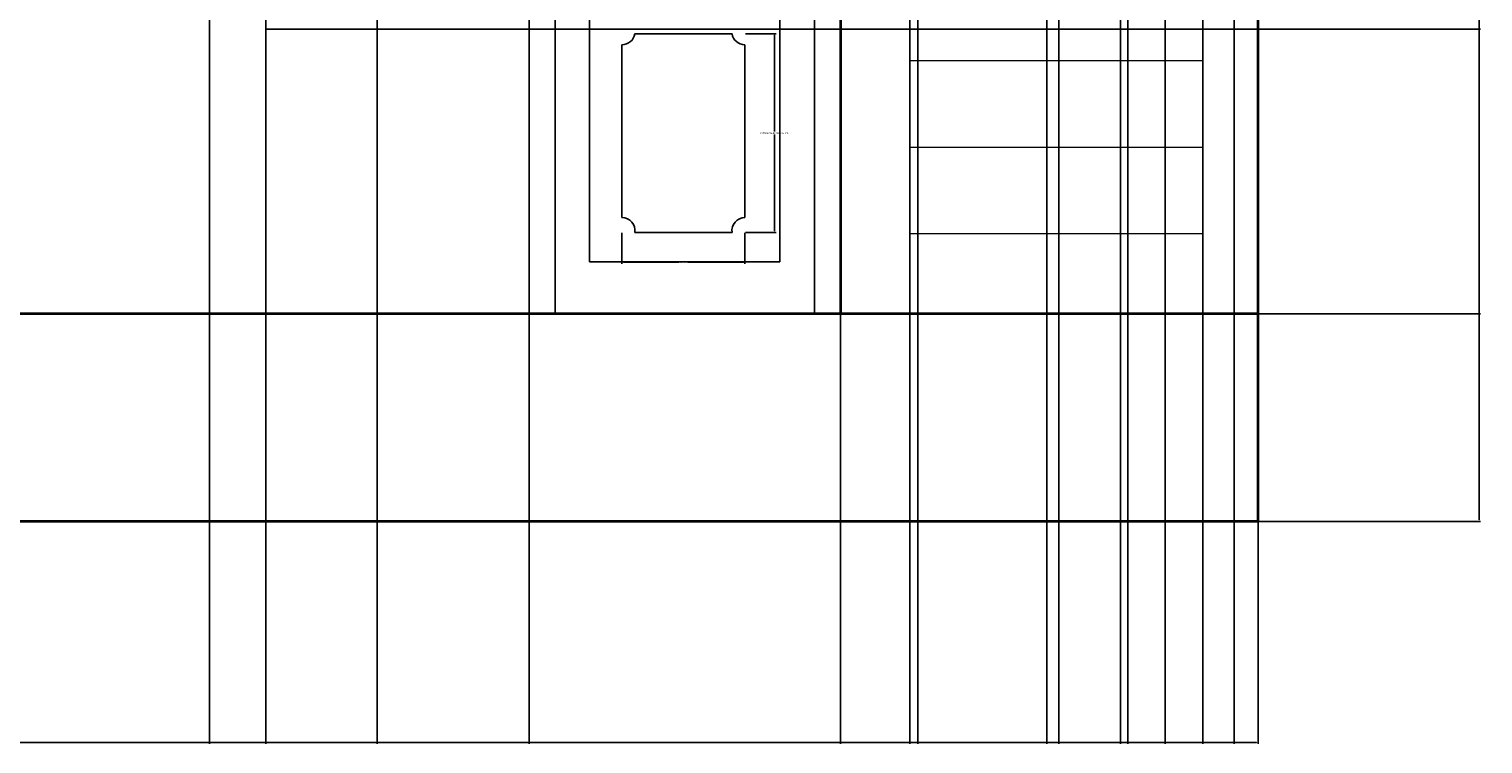
# Model space of a CAD drawing. Units: inches. Extents: x 93 to 565, y 123 to 656.
# Tile 3 of 18: x 397 to 565, y 134 to 217. Entities that reach past the tile are written whole.
import ezdxf

# ---------------------------------------------------------------- set-up
doc = ezdxf.new("R2010")
doc.units = ezdxf.units.IN
doc.header["$MEASUREMENT"] = 0
for name, color, linetype, lineweight in [('A-ANNO-DIMS', 2, 'Continuous', 18), ('A-DOOR', 3, 'Continuous', 25), ('A-ELEV', 7, 'Continuous', 35), ('A-FLOR-STRS', 6, 'Continuous', 18)]:
    doc.layers.add(name, color=color, linetype=linetype, lineweight=lineweight)
doc.styles.get("Standard").update_dxf_attribs({"font": 'arial.ttf'})
doc.dimstyles.get("Standard").update_dxf_attribs({"dimtxt": 0.18, "dimasz": 0.18, "dimexe": 0.18, "dimexo": 0.0625, "dimgap": 0.09, "dimtad": 0, "dimtih": 1, "dimtoh": 1, "dimdec": 4, "dimzin": 0, "dimdsep": 46, "dimtxsty": 'Standard', "dimcen": 0.09, "dimadec": 0, "dimazin": 0, "dimtfac": 1, "dimtdec": 4, "dimtofl": 0, "dimtmove": 0, "dimatfit": 3, "dimfxl": 1, "dimtolj": 1, "dimtzin": 0, "dimarcsym": 0})

# ---------------------------------------------------------------- blocks, each defined once
blk = doc.blocks.new('*U4')
blk.add_lwpolyline([(3.12, 0.01), (0.12, 0.01), (0.12, 84.01), (36.12, 84.01), (36.12, 0.01), (33.12, 0.01)])
for points in [[(33.12, 80.99), (33.12, 0.01), (3.12, 0.01), (3.12, 80.99)], [(29.12, 6.01), (29.12, 74.99), (7.12, 74.99), (7.12, 6.01)]]:
    blk.add_lwpolyline(points, close=True)
blk.add_circle((31.12, 42.01), 1)
blk = doc.blocks.new('DOOR-PANEL-LOWER')
for points in [[(1.48, 22.97), (12.73, 22.97)], [(0, 1.72), (0, 21.69)], [(14.21, 21.69), (14.21, 1.72)], [(12.73, 0), (1.48, 0)]]:
    blk.add_lwpolyline(points)
for centre, start, end in [((0, 23.19), 270, 351.5859), ((14.21, 23.19), 188.4141, 270), ((0, 0.22), 351.5859, 90), ((14.21, 0.22), 90, 188.4141)]:
    blk.add_arc(centre, 1.5, start, end)
blk = doc.blocks.new('*D24')
at = {"layer": 'A-ANNO-DIMS', "color": 0, "lineweight": -2, "transparency": 16777216}
for p, q in [((479.78, 216.1), (483.34, 216.1)), ((483.16, 215.92), (483.16, 204.79)), ((483.16, 193.3), (483.16, 204.43)), ((479.78, 193.12), (483.34, 193.12))]:
    blk.add_line(p, q, dxfattribs=at)
at = {"layer": 'A-ANNO-DIMS', "color": 0, "transparency": 16777216}
for points in [[(483.13, 215.92), (483.19, 215.92), (483.16, 216.1)], [(483.13, 193.3), (483.19, 193.3), (483.16, 193.12)]]:
    blk.add_solid(points, dxfattribs=at)
at = {"layer": 'Defpoints', "color": 0, "transparency": 16777216}
for p in [(479.72, 216.1), (483.16, 216.1), (479.72, 193.12)]:
    blk.add_point(p, dxfattribs=at)
at = {"layer": 'A-ANNO-DIMS', "color": 0, "transparency": 16777216, "insert": (483.16, 204.61), "char_height": 0.18, "attachment_point": 5}
blk.add_mtext('\\A1;DOOR LOWER PANEL 23 TYP.', dxfattribs=at)
blk = doc.blocks.new('*D25')
at = {"layer": 'A-ANNO-DIMS', "color": 0, "lineweight": -2, "transparency": 16777216}
for p, q in [((465.5, 193.06), (465.5, 189.5)), ((479.72, 193.06), (479.72, 189.5)), ((465.68, 189.68), (472.09, 189.68)), ((479.54, 189.68), (473.13, 189.68))]:
    blk.add_line(p, q, dxfattribs=at)
at = {"layer": 'A-ANNO-DIMS', "color": 0, "transparency": 16777216}
for points in [[(465.68, 189.71), (465.68, 189.65), (465.5, 189.68)], [(479.54, 189.71), (479.54, 189.65), (479.72, 189.68)]]:
    blk.add_solid(points, dxfattribs=at)
at = {"layer": 'Defpoints', "color": 0, "transparency": 16777216}
for p in [(465.5, 193.12), (479.72, 193.12), (479.72, 189.68)]:
    blk.add_point(p, dxfattribs=at)
at = {"layer": 'A-ANNO-DIMS', "color": 0, "transparency": 16777216, "insert": (472.61, 189.68), "char_height": 0.18, "attachment_point": 5}
blk.add_mtext('\\A1;14 TYP.', dxfattribs=at)
blk = doc.blocks.new('*D29')
at = {"layer": 'A-ANNO-DIMS', "color": 0, "lineweight": -2, "transparency": 16777216}
for p, q in [((437.19, 594.34), (437.19, 134)), ((295.69, 183.67), (295.69, 134)), ((295.87, 134.18), (366.05, 134.18)), ((437.01, 134.18), (366.82, 134.18))]:
    blk.add_line(p, q, dxfattribs=at)
at = {"layer": 'A-ANNO-DIMS', "color": 0, "transparency": 16777216}
for points in [[(295.87, 134.21), (295.87, 134.15), (295.69, 134.18)], [(437.01, 134.21), (437.01, 134.15), (437.19, 134.18)]]:
    blk.add_solid(points, dxfattribs=at)
at = {"layer": 'Defpoints', "color": 0, "transparency": 16777216}
for p in [(437.19, 594.4), (295.69, 183.73), (437.19, 134.18)]:
    blk.add_point(p, dxfattribs=at)
at = {"layer": 'A-ANNO-DIMS', "color": 0, "transparency": 16777216, "insert": (366.44, 134.18), "char_height": 0.18, "attachment_point": 5}
blk.add_mtext('\\A1;141.5', dxfattribs=at)
blk = doc.blocks.new('*D30')
at = {"layer": 'A-ANNO-DIMS', "color": 0, "lineweight": -2, "transparency": 16777216}
for p, q in [((437.19, 594.34), (437.19, 134)), ((539.08, 159.67), (539.08, 134)), ((437.37, 134.18), (487.75, 134.18)), ((538.9, 134.18), (488.52, 134.18))]:
    blk.add_line(p, q, dxfattribs=at)
at = {"layer": 'A-ANNO-DIMS', "color": 0, "transparency": 16777216}
for points in [[(437.37, 134.21), (437.37, 134.15), (437.19, 134.18)], [(538.9, 134.21), (538.9, 134.15), (539.08, 134.18)]]:
    blk.add_solid(points, dxfattribs=at)
at = {"layer": 'Defpoints', "color": 0, "transparency": 16777216}
for p in [(437.19, 594.4), (539.08, 159.73), (539.08, 134.18)]:
    blk.add_point(p, dxfattribs=at)
at = {"layer": 'A-ANNO-DIMS', "color": 0, "transparency": 16777216, "insert": (488.13, 134.18), "char_height": 0.18, "attachment_point": 5}
blk.add_mtext('\\A1;101.9', dxfattribs=at)
blk = doc.blocks.new('*D31')
at = {"layer": 'A-ANNO-DIMS', "color": 0, "lineweight": -2, "transparency": 16777216}
for p, q in [((417.87, 630.4), (564.81, 630.4)), ((564.63, 630.22), (564.63, 395.25)), ((564.63, 159.91), (564.63, 394.89)), ((119.14, 159.73), (564.81, 159.73))]:
    blk.add_line(p, q, dxfattribs=at)
at = {"layer": 'A-ANNO-DIMS', "color": 0, "transparency": 16777216}
for points in [[(564.6, 630.22), (564.66, 630.22), (564.63, 630.4)], [(564.6, 159.91), (564.66, 159.91), (564.63, 159.73)]]:
    blk.add_solid(points, dxfattribs=at)
at = {"layer": 'Defpoints', "color": 0, "transparency": 16777216}
for p in [(417.81, 630.4), (564.63, 630.4), (119.08, 159.73)]:
    blk.add_point(p, dxfattribs=at)
at = {"layer": 'A-ANNO-DIMS', "color": 0, "transparency": 16777216, "insert": (564.63, 395.07), "char_height": 0.18, "attachment_point": 5}
blk.add_mtext('\\A1;470.7', dxfattribs=at)
blk = doc.blocks.new('*D56')
at = {"layer": 'A-ANNO-DIMS', "color": 0, "lineweight": -2, "transparency": 16777216}
for p, q in [((309.74, 275.71), (309.74, 134)), ((424.3, 275.71), (424.3, 134)), ((309.92, 134.18), (366.57, 134.18)), ((424.12, 134.18), (367.48, 134.18))]:
    blk.add_line(p, q, dxfattribs=at)
at = {"layer": 'A-ANNO-DIMS', "color": 0, "transparency": 16777216}
for points in [[(309.92, 134.21), (309.92, 134.15), (309.74, 134.18)], [(424.12, 134.21), (424.12, 134.15), (424.3, 134.18)]]:
    blk.add_solid(points, dxfattribs=at)
at = {"layer": 'Defpoints', "color": 0, "transparency": 16777216}
for p in [(309.74, 275.77), (424.3, 275.77), (424.3, 134.18)]:
    blk.add_point(p, dxfattribs=at)
at = {"layer": 'A-ANNO-DIMS', "color": 0, "transparency": 16777216, "insert": (367.02, 134.18), "char_height": 0.18, "attachment_point": 5}
blk.add_mtext('\\A1;114.56', dxfattribs=at)
blk = doc.blocks.new('*D57')
at = {"layer": 'A-ANNO-DIMS', "color": 0, "lineweight": -2, "transparency": 16777216}
for p, q in [((424.37, 275.77), (564.81, 275.77)), ((564.63, 275.59), (564.63, 246.38)), ((564.63, 216.81), (564.63, 246.02)), ((424.37, 216.63), (564.81, 216.63))]:
    blk.add_line(p, q, dxfattribs=at)
at = {"layer": 'A-ANNO-DIMS', "color": 0, "transparency": 16777216}
for points in [[(564.6, 275.59), (564.66, 275.59), (564.63, 275.77)], [(564.6, 216.81), (564.66, 216.81), (564.63, 216.63)]]:
    blk.add_solid(points, dxfattribs=at)
at = {"layer": 'Defpoints', "color": 0, "transparency": 16777216}
for p in [(424.3, 275.77), (564.63, 275.77), (424.3, 216.63)]:
    blk.add_point(p, dxfattribs=at)
at = {"layer": 'A-ANNO-DIMS', "color": 0, "transparency": 16777216, "insert": (564.63, 246.2), "char_height": 0.18, "attachment_point": 5}
blk.add_mtext('\\A1;59.14', dxfattribs=at)
blk = doc.blocks.new('*D59')
at = {"layer": 'A-ANNO-DIMS', "color": 0, "lineweight": -2, "transparency": 16777216}
for p, q in [((454.77, 267.67), (454.77, 134)), ((490.77, 267.67), (490.77, 134)), ((454.95, 134.18), (472.55, 134.18)), ((490.59, 134.18), (472.99, 134.18))]:
    blk.add_line(p, q, dxfattribs=at)
at = {"layer": 'A-ANNO-DIMS', "color": 0, "transparency": 16777216}
for points in [[(454.95, 134.21), (454.95, 134.15), (454.77, 134.18)], [(490.59, 134.21), (490.59, 134.15), (490.77, 134.18)]]:
    blk.add_solid(points, dxfattribs=at)
at = {"layer": 'Defpoints', "color": 0, "transparency": 16777216}
for p in [(454.77, 267.73), (490.77, 267.73), (490.77, 134.18)]:
    blk.add_point(p, dxfattribs=at)
at = {"layer": 'A-ANNO-DIMS', "color": 0, "transparency": 16777216, "insert": (472.77, 134.18), "char_height": 0.18, "attachment_point": 5}
blk.add_mtext('\\A1;36', dxfattribs=at)
blk = doc.blocks.new('*D60')
at = {"layer": 'A-ANNO-DIMS', "color": 0, "lineweight": -2, "transparency": 16777216}
for p, q in [((490.83, 267.73), (564.81, 267.73)), ((564.63, 267.55), (564.63, 225.91)), ((564.63, 183.91), (564.63, 225.55)), ((490.83, 183.73), (564.81, 183.73))]:
    blk.add_line(p, q, dxfattribs=at)
at = {"layer": 'A-ANNO-DIMS', "color": 0, "transparency": 16777216}
for points in [[(564.6, 267.55), (564.66, 267.55), (564.63, 267.73)], [(564.6, 183.91), (564.66, 183.91), (564.63, 183.73)]]:
    blk.add_solid(points, dxfattribs=at)
at = {"layer": 'Defpoints', "color": 0, "transparency": 16777216}
for p in [(490.77, 267.73), (564.63, 267.73), (490.77, 183.73)]:
    blk.add_point(p, dxfattribs=at)
at = {"layer": 'A-ANNO-DIMS', "color": 0, "transparency": 16777216, "insert": (564.63, 225.73), "char_height": 0.18, "attachment_point": 5}
blk.add_mtext('\\A1;84', dxfattribs=at)
blk = doc.blocks.new('*D61')
at = {"layer": 'A-ANNO-DIMS', "color": 0, "lineweight": -2, "transparency": 16777216}
for p, q in [((424.3, 216.57), (424.3, 134)), ((454.77, 183.67), (454.77, 134)), ((424.48, 134.18), (439.07, 134.18)), ((454.59, 134.18), (440, 134.18))]:
    blk.add_line(p, q, dxfattribs=at)
at = {"layer": 'A-ANNO-DIMS', "color": 0, "transparency": 16777216}
for points in [[(424.48, 134.21), (424.48, 134.15), (424.3, 134.18)], [(454.59, 134.21), (454.59, 134.15), (454.77, 134.18)]]:
    blk.add_solid(points, dxfattribs=at)
at = {"layer": 'Defpoints', "color": 0, "transparency": 16777216}
for p in [(424.3, 216.63), (454.77, 183.73), (454.77, 134.18)]:
    blk.add_point(p, dxfattribs=at)
at = {"layer": 'A-ANNO-DIMS', "color": 0, "transparency": 16777216, "insert": (439.54, 134.18), "char_height": 0.18, "attachment_point": 5}
blk.add_mtext('\\A1;30.466', dxfattribs=at)
blk = doc.blocks.new('*D62')
at = {"layer": 'A-ANNO-DIMS', "color": 0, "lineweight": -2, "transparency": 16777216}
for p, q in [((498.79, 312.92), (498.79, 134)), ((532.69, 312.92), (532.69, 134)), ((498.97, 134.18), (515.42, 134.18)), ((532.51, 134.18), (516.07, 134.18))]:
    blk.add_line(p, q, dxfattribs=at)
at = {"layer": 'A-ANNO-DIMS', "color": 0, "transparency": 16777216}
for points in [[(498.97, 134.21), (498.97, 134.15), (498.79, 134.18)], [(532.51, 134.21), (532.51, 134.15), (532.69, 134.18)]]:
    blk.add_solid(points, dxfattribs=at)
at = {"layer": 'Defpoints', "color": 0, "transparency": 16777216}
for p in [(498.79, 312.99), (532.69, 312.99), (532.69, 134.18)]:
    blk.add_point(p, dxfattribs=at)
at = {"layer": 'A-ANNO-DIMS', "color": 0, "transparency": 16777216, "insert": (515.74, 134.18), "char_height": 0.18, "attachment_point": 5}
blk.add_mtext('\\A1;33.9', dxfattribs=at)
blk = doc.blocks.new('*D90')
at = {"layer": 'A-ANNO-DIMS', "color": 0, "lineweight": -2, "transparency": 16777216}
for p, q in [((417.81, 594.34), (417.81, 134)), ((437.19, 594.34), (437.19, 134)), ((417.99, 134.18), (427.11, 134.18)), ((437.01, 134.18), (427.88, 134.18))]:
    blk.add_line(p, q, dxfattribs=at)
at = {"layer": 'A-ANNO-DIMS', "color": 0, "transparency": 16777216}
for points in [[(417.99, 134.21), (417.99, 134.15), (417.81, 134.18)], [(437.01, 134.21), (437.01, 134.15), (437.19, 134.18)]]:
    blk.add_solid(points, dxfattribs=at)
at = {"layer": 'Defpoints', "color": 0, "transparency": 16777216}
for p in [(417.81, 594.4), (437.19, 594.4), (437.19, 134.18)]:
    blk.add_point(p, dxfattribs=at)
at = {"layer": 'A-ANNO-DIMS', "color": 0, "transparency": 16777216, "insert": (427.5, 134.18), "char_height": 0.18, "attachment_point": 5}
blk.add_mtext('\\A1;19.38', dxfattribs=at)
blk = doc.blocks.new('*D91')
at = {"layer": 'A-ANNO-DIMS', "color": 0, "lineweight": -2, "transparency": 16777216}
for p, q in [((499.73, 599.75), (499.73, 134)), ((437.19, 594.34), (437.19, 134)), ((437.37, 134.18), (468.07, 134.18)), ((499.55, 134.18), (468.85, 134.18))]:
    blk.add_line(p, q, dxfattribs=at)
at = {"layer": 'A-ANNO-DIMS', "color": 0, "transparency": 16777216}
for points in [[(437.37, 134.21), (437.37, 134.15), (437.19, 134.18)], [(499.55, 134.21), (499.55, 134.15), (499.73, 134.18)]]:
    blk.add_solid(points, dxfattribs=at)
at = {"layer": 'Defpoints', "color": 0, "transparency": 16777216}
for p in [(499.73, 599.82), (437.19, 594.4), (499.73, 134.18)]:
    blk.add_point(p, dxfattribs=at)
at = {"layer": 'A-ANNO-DIMS', "color": 0, "transparency": 16777216, "insert": (468.46, 134.18), "char_height": 0.18, "attachment_point": 5}
blk.add_mtext('\\A1;62.54', dxfattribs=at)
blk = doc.blocks.new('*D92')
at = {"layer": 'A-ANNO-DIMS', "color": 0, "lineweight": -2, "transparency": 16777216}
for p, q in [((523.14, 603.14), (523.14, 134)), ((499.73, 599.75), (499.73, 134)), ((499.91, 134.18), (510.97, 134.18)), ((522.96, 134.18), (511.9, 134.18))]:
    blk.add_line(p, q, dxfattribs=at)
at = {"layer": 'A-ANNO-DIMS', "color": 0, "transparency": 16777216}
for points in [[(499.91, 134.21), (499.91, 134.15), (499.73, 134.18)], [(522.96, 134.21), (522.96, 134.15), (523.14, 134.18)]]:
    blk.add_solid(points, dxfattribs=at)
at = {"layer": 'Defpoints', "color": 0, "transparency": 16777216}
for p in [(523.14, 603.2), (499.73, 599.82), (523.14, 134.18)]:
    blk.add_point(p, dxfattribs=at)
at = {"layer": 'A-ANNO-DIMS', "color": 0, "transparency": 16777216, "insert": (511.44, 134.18), "char_height": 0.18, "attachment_point": 5}
blk.add_mtext('\\A1;23.412', dxfattribs=at)
blk = doc.blocks.new('*D93')
at = {"layer": 'A-ANNO-DIMS', "color": 0, "lineweight": -2, "transparency": 16777216}
for p, q in [((523.14, 603.14), (523.14, 134)), ((539.08, 594.34), (539.08, 134)), ((523.32, 134.18), (530.66, 134.18)), ((538.9, 134.18), (531.57, 134.18))]:
    blk.add_line(p, q, dxfattribs=at)
at = {"layer": 'A-ANNO-DIMS', "color": 0, "transparency": 16777216}
for points in [[(523.32, 134.21), (523.32, 134.15), (523.14, 134.18)], [(538.9, 134.21), (538.9, 134.15), (539.08, 134.18)]]:
    blk.add_solid(points, dxfattribs=at)
at = {"layer": 'Defpoints', "color": 0, "transparency": 16777216}
for p in [(523.14, 603.2), (539.08, 594.4), (539.08, 134.18)]:
    blk.add_point(p, dxfattribs=at)
at = {"layer": 'A-ANNO-DIMS', "color": 0, "transparency": 16777216, "insert": (531.11, 134.18), "char_height": 0.18, "attachment_point": 5}
blk.add_mtext('\\A1;15.938', dxfattribs=at)
blk = doc.blocks.new('*D108')
at = {"layer": 'A-ANNO-DIMS', "color": 0, "lineweight": -2, "transparency": 16777216}
for p, q in [((437.19, 594.34), (437.19, 134)), ((295.69, 183.67), (295.69, 134)), ((295.87, 134.18), (365.93, 134.18)), ((437.01, 134.18), (366.95, 134.18))]:
    blk.add_line(p, q, dxfattribs=at)
at = {"layer": 'A-ANNO-DIMS', "color": 0, "transparency": 16777216}
for points in [[(295.87, 134.21), (295.87, 134.15), (295.69, 134.18)], [(437.01, 134.21), (437.01, 134.15), (437.19, 134.18)]]:
    blk.add_solid(points, dxfattribs=at)
at = {"layer": 'Defpoints', "color": 0, "transparency": 16777216}
for p in [(437.19, 594.4), (295.69, 183.73), (437.19, 134.18)]:
    blk.add_point(p, dxfattribs=at)
at = {"layer": 'A-ANNO-DIMS', "color": 0, "transparency": 16777216, "insert": (366.44, 134.18), "char_height": 0.18, "attachment_point": 5}
blk.add_mtext('\\A1;141.501', dxfattribs=at)
blk = doc.blocks.new('*D109')
at = {"layer": 'A-ANNO-DIMS', "color": 0, "lineweight": -2, "transparency": 16777216}
for p, q in [((437.19, 594.34), (437.19, 134)), ((539.08, 159.67), (539.08, 134)), ((437.37, 134.18), (487.63, 134.18)), ((538.9, 134.18), (488.64, 134.18))]:
    blk.add_line(p, q, dxfattribs=at)
at = {"layer": 'A-ANNO-DIMS', "color": 0, "transparency": 16777216}
for points in [[(437.37, 134.21), (437.37, 134.15), (437.19, 134.18)], [(538.9, 134.21), (538.9, 134.15), (539.08, 134.18)]]:
    blk.add_solid(points, dxfattribs=at)
at = {"layer": 'Defpoints', "color": 0, "transparency": 16777216}
for p in [(437.19, 594.4), (539.08, 159.73), (539.08, 134.18)]:
    blk.add_point(p, dxfattribs=at)
at = {"layer": 'A-ANNO-DIMS', "color": 0, "transparency": 16777216, "insert": (488.13, 134.18), "char_height": 0.18, "attachment_point": 5}
blk.add_mtext('\\A1;101.891', dxfattribs=at)
blk = doc.blocks.new('*D110')
at = {"layer": 'A-ANNO-DIMS', "color": 0, "lineweight": -2, "transparency": 16777216}
for p, q in [((417.87, 630.4), (564.81, 630.4)), ((564.63, 630.22), (564.63, 395.25)), ((564.63, 159.91), (564.63, 394.89)), ((119.14, 159.73), (564.81, 159.73))]:
    blk.add_line(p, q, dxfattribs=at)
at = {"layer": 'A-ANNO-DIMS', "color": 0, "transparency": 16777216}
for points in [[(564.6, 630.22), (564.66, 630.22), (564.63, 630.4)], [(564.6, 159.91), (564.66, 159.91), (564.63, 159.73)]]:
    blk.add_solid(points, dxfattribs=at)
at = {"layer": 'Defpoints', "color": 0, "transparency": 16777216}
for p in [(417.81, 630.4), (564.63, 630.4), (119.08, 159.73)]:
    blk.add_point(p, dxfattribs=at)
at = {"layer": 'A-ANNO-DIMS', "color": 0, "transparency": 16777216, "insert": (564.63, 395.07), "char_height": 0.18, "attachment_point": 5}
blk.add_mtext('\\A1;470.673', dxfattribs=at)
blk = doc.blocks.new('*D135')
at = {"layer": 'A-ANNO-DIMS', "color": 0, "lineweight": -2, "transparency": 16777216}
for p, q in [((309.74, 275.71), (309.74, 134)), ((424.3, 275.71), (424.3, 134)), ((309.92, 134.18), (366.5, 134.18)), ((424.12, 134.18), (367.55, 134.18))]:
    blk.add_line(p, q, dxfattribs=at)
at = {"layer": 'A-ANNO-DIMS', "color": 0, "transparency": 16777216}
for points in [[(309.92, 134.21), (309.92, 134.15), (309.74, 134.18)], [(424.12, 134.21), (424.12, 134.15), (424.3, 134.18)]]:
    blk.add_solid(points, dxfattribs=at)
at = {"layer": 'Defpoints', "color": 0, "transparency": 16777216}
for p in [(309.74, 275.77), (424.3, 275.77), (424.3, 134.18)]:
    blk.add_point(p, dxfattribs=at)
at = {"layer": 'A-ANNO-DIMS', "color": 0, "transparency": 16777216, "insert": (367.02, 134.18), "char_height": 0.18, "attachment_point": 5}
blk.add_mtext('\\A1;114.560', dxfattribs=at)
blk = doc.blocks.new('*D136')
at = {"layer": 'A-ANNO-DIMS', "color": 0, "lineweight": -2, "transparency": 16777216}
for p, q in [((424.37, 275.77), (564.81, 275.77)), ((564.63, 275.59), (564.63, 246.38)), ((564.63, 216.81), (564.63, 246.02)), ((424.37, 216.63), (564.81, 216.63))]:
    blk.add_line(p, q, dxfattribs=at)
at = {"layer": 'A-ANNO-DIMS', "color": 0, "transparency": 16777216}
for points in [[(564.6, 275.59), (564.66, 275.59), (564.63, 275.77)], [(564.6, 216.81), (564.66, 216.81), (564.63, 216.63)]]:
    blk.add_solid(points, dxfattribs=at)
at = {"layer": 'Defpoints', "color": 0, "transparency": 16777216}
for p in [(424.3, 275.77), (564.63, 275.77), (424.3, 216.63)]:
    blk.add_point(p, dxfattribs=at)
at = {"layer": 'A-ANNO-DIMS', "color": 0, "transparency": 16777216, "insert": (564.63, 246.2), "char_height": 0.18, "attachment_point": 5}
blk.add_mtext('\\A1;59.144', dxfattribs=at)
blk = doc.blocks.new('*D138')
at = {"layer": 'A-ANNO-DIMS', "color": 0, "lineweight": -2, "transparency": 16777216}
for p, q in [((454.77, 267.67), (454.77, 134)), ((490.77, 267.67), (490.77, 134)), ((454.95, 134.18), (472.31, 134.18)), ((490.59, 134.18), (473.23, 134.18))]:
    blk.add_line(p, q, dxfattribs=at)
at = {"layer": 'A-ANNO-DIMS', "color": 0, "transparency": 16777216}
for points in [[(454.95, 134.21), (454.95, 134.15), (454.77, 134.18)], [(490.59, 134.21), (490.59, 134.15), (490.77, 134.18)]]:
    blk.add_solid(points, dxfattribs=at)
at = {"layer": 'Defpoints', "color": 0, "transparency": 16777216}
for p in [(454.77, 267.73), (490.77, 267.73), (490.77, 134.18)]:
    blk.add_point(p, dxfattribs=at)
at = {"layer": 'A-ANNO-DIMS', "color": 0, "transparency": 16777216, "insert": (472.77, 134.18), "char_height": 0.18, "attachment_point": 5}
blk.add_mtext('\\A1;36.000', dxfattribs=at)
blk = doc.blocks.new('*D139')
at = {"layer": 'A-ANNO-DIMS', "color": 0, "lineweight": -2, "transparency": 16777216}
for p, q in [((490.83, 267.73), (564.81, 267.73)), ((564.63, 267.55), (564.63, 225.91)), ((564.63, 183.91), (564.63, 225.55)), ((490.83, 183.73), (564.81, 183.73))]:
    blk.add_line(p, q, dxfattribs=at)
at = {"layer": 'A-ANNO-DIMS', "color": 0, "transparency": 16777216}
for points in [[(564.6, 267.55), (564.66, 267.55), (564.63, 267.73)], [(564.6, 183.91), (564.66, 183.91), (564.63, 183.73)]]:
    blk.add_solid(points, dxfattribs=at)
at = {"layer": 'Defpoints', "color": 0, "transparency": 16777216}
for p in [(490.77, 267.73), (564.63, 267.73), (490.77, 183.73)]:
    blk.add_point(p, dxfattribs=at)
at = {"layer": 'A-ANNO-DIMS', "color": 0, "transparency": 16777216, "insert": (564.63, 225.73), "char_height": 0.18, "attachment_point": 5}
blk.add_mtext('\\A1;84.000', dxfattribs=at)
blk = doc.blocks.new('*D140')
at = {"layer": 'A-ANNO-DIMS', "color": 0, "lineweight": -2, "transparency": 16777216}
for p, q in [((424.3, 216.57), (424.3, 134)), ((454.77, 183.67), (454.77, 134)), ((424.48, 134.18), (439.07, 134.18)), ((454.59, 134.18), (440, 134.18))]:
    blk.add_line(p, q, dxfattribs=at)
at = {"layer": 'A-ANNO-DIMS', "color": 0, "transparency": 16777216}
for points in [[(424.48, 134.21), (424.48, 134.15), (424.3, 134.18)], [(454.59, 134.21), (454.59, 134.15), (454.77, 134.18)]]:
    blk.add_solid(points, dxfattribs=at)
at = {"layer": 'Defpoints', "color": 0, "transparency": 16777216}
for p in [(424.3, 216.63), (454.77, 183.73), (454.77, 134.18)]:
    blk.add_point(p, dxfattribs=at)
at = {"layer": 'A-ANNO-DIMS', "color": 0, "transparency": 16777216, "insert": (439.54, 134.18), "char_height": 0.18, "attachment_point": 5}
blk.add_mtext('\\A1;30.466', dxfattribs=at)
blk = doc.blocks.new('*D141')
at = {"layer": 'A-ANNO-DIMS', "color": 0, "lineweight": -2, "transparency": 16777216}
for p, q in [((498.79, 312.92), (498.79, 134)), ((532.69, 312.92), (532.69, 134)), ((498.97, 134.18), (515.28, 134.18)), ((532.51, 134.18), (516.21, 134.18))]:
    blk.add_line(p, q, dxfattribs=at)
at = {"layer": 'A-ANNO-DIMS', "color": 0, "transparency": 16777216}
for points in [[(498.97, 134.21), (498.97, 134.15), (498.79, 134.18)], [(532.51, 134.21), (532.51, 134.15), (532.69, 134.18)]]:
    blk.add_solid(points, dxfattribs=at)
at = {"layer": 'Defpoints', "color": 0, "transparency": 16777216}
for p in [(498.79, 312.99), (532.69, 312.99), (532.69, 134.18)]:
    blk.add_point(p, dxfattribs=at)
at = {"layer": 'A-ANNO-DIMS', "color": 0, "transparency": 16777216, "insert": (515.74, 134.18), "char_height": 0.18, "attachment_point": 5}
blk.add_mtext('\\A1;33.897', dxfattribs=at)
blk = doc.blocks.new('*D169')
at = {"layer": 'A-ANNO-DIMS', "color": 0, "lineweight": -2, "transparency": 16777216}
for p, q in [((417.81, 594.34), (417.81, 134)), ((437.19, 594.34), (437.19, 134)), ((417.99, 134.18), (427.04, 134.18)), ((437.01, 134.18), (427.95, 134.18))]:
    blk.add_line(p, q, dxfattribs=at)
at = {"layer": 'A-ANNO-DIMS', "color": 0, "transparency": 16777216}
for points in [[(417.99, 134.21), (417.99, 134.15), (417.81, 134.18)], [(437.01, 134.21), (437.01, 134.15), (437.19, 134.18)]]:
    blk.add_solid(points, dxfattribs=at)
at = {"layer": 'Defpoints', "color": 0, "transparency": 16777216}
for p in [(417.81, 594.4), (437.19, 594.4), (437.19, 134.18)]:
    blk.add_point(p, dxfattribs=at)
at = {"layer": 'A-ANNO-DIMS', "color": 0, "transparency": 16777216, "insert": (427.5, 134.18), "char_height": 0.18, "attachment_point": 5}
blk.add_mtext('\\A1;19.379', dxfattribs=at)
blk = doc.blocks.new('*D170')
at = {"layer": 'A-ANNO-DIMS', "color": 0, "lineweight": -2, "transparency": 16777216}
for p, q in [((499.73, 599.75), (499.73, 134)), ((437.19, 594.34), (437.19, 134)), ((437.37, 134.18), (468.01, 134.18)), ((499.55, 134.18), (468.91, 134.18))]:
    blk.add_line(p, q, dxfattribs=at)
at = {"layer": 'A-ANNO-DIMS', "color": 0, "transparency": 16777216}
for points in [[(437.37, 134.21), (437.37, 134.15), (437.19, 134.18)], [(499.55, 134.21), (499.55, 134.15), (499.73, 134.18)]]:
    blk.add_solid(points, dxfattribs=at)
at = {"layer": 'Defpoints', "color": 0, "transparency": 16777216}
for p in [(499.73, 599.82), (437.19, 594.4), (499.73, 134.18)]:
    blk.add_point(p, dxfattribs=at)
at = {"layer": 'A-ANNO-DIMS', "color": 0, "transparency": 16777216, "insert": (468.46, 134.18), "char_height": 0.18, "attachment_point": 5}
blk.add_mtext('\\A1;62.541', dxfattribs=at)
blk = doc.blocks.new('*D171')
at = {"layer": 'A-ANNO-DIMS', "color": 0, "lineweight": -2, "transparency": 16777216}
for p, q in [((523.14, 603.14), (523.14, 134)), ((499.73, 599.75), (499.73, 134)), ((499.91, 134.18), (510.97, 134.18)), ((522.96, 134.18), (511.9, 134.18))]:
    blk.add_line(p, q, dxfattribs=at)
at = {"layer": 'A-ANNO-DIMS', "color": 0, "transparency": 16777216}
for points in [[(499.91, 134.21), (499.91, 134.15), (499.73, 134.18)], [(522.96, 134.21), (522.96, 134.15), (523.14, 134.18)]]:
    blk.add_solid(points, dxfattribs=at)
at = {"layer": 'Defpoints', "color": 0, "transparency": 16777216}
for p in [(523.14, 603.2), (499.73, 599.82), (523.14, 134.18)]:
    blk.add_point(p, dxfattribs=at)
at = {"layer": 'A-ANNO-DIMS', "color": 0, "transparency": 16777216, "insert": (511.44, 134.18), "char_height": 0.18, "attachment_point": 5}
blk.add_mtext('\\A1;23.412', dxfattribs=at)
blk = doc.blocks.new('*D172')
at = {"layer": 'A-ANNO-DIMS', "color": 0, "lineweight": -2, "transparency": 16777216}
for p, q in [((523.14, 603.14), (523.14, 134)), ((539.08, 594.34), (539.08, 134)), ((523.32, 134.18), (530.66, 134.18)), ((538.9, 134.18), (531.57, 134.18))]:
    blk.add_line(p, q, dxfattribs=at)
at = {"layer": 'A-ANNO-DIMS', "color": 0, "transparency": 16777216}
for points in [[(523.32, 134.21), (523.32, 134.15), (523.14, 134.18)], [(538.9, 134.21), (538.9, 134.15), (539.08, 134.18)]]:
    blk.add_solid(points, dxfattribs=at)
at = {"layer": 'Defpoints', "color": 0, "transparency": 16777216}
for p in [(523.14, 603.2), (539.08, 594.4), (539.08, 134.18)]:
    blk.add_point(p, dxfattribs=at)
at = {"layer": 'A-ANNO-DIMS', "color": 0, "transparency": 16777216, "insert": (531.11, 134.18), "char_height": 0.18, "attachment_point": 5}
blk.add_mtext('\\A1;15.938', dxfattribs=at)
blk = doc.blocks.new('*D180')
at = {"layer": 'A-ANNO-DIMS', "color": 0, "lineweight": -2, "transparency": 16777216}
for p, q in [((514.64, 348.49), (514.64, 134)), ((516.01, 331.37), (516.01, 134)), ((514.82, 134.18), (514.94, 134.18)), ((515.83, 134.18), (515.71, 134.18))]:
    blk.add_line(p, q, dxfattribs=at)
at = {"layer": 'A-ANNO-DIMS', "color": 0, "transparency": 16777216}
for points in [[(514.82, 134.21), (514.82, 134.15), (514.64, 134.18)], [(515.83, 134.21), (515.83, 134.15), (516.01, 134.18)]]:
    blk.add_solid(points, dxfattribs=at)
at = {"layer": 'Defpoints', "color": 0, "transparency": 16777216}
for p in [(514.64, 348.55), (516.01, 331.43), (516.01, 134.18)]:
    blk.add_point(p, dxfattribs=at)
at = {"layer": 'A-ANNO-DIMS', "color": 0, "transparency": 16777216, "insert": (515.33, 134.18), "char_height": 0.18, "attachment_point": 5}
blk.add_mtext('\\A1;1.367', dxfattribs=at)
blk = doc.blocks.new('*D181')
at = {"layer": 'A-ANNO-DIMS', "color": 0, "lineweight": -2, "transparency": 16777216}
for p, q in [((516.01, 331.37), (516.01, 134)), ((524.02, 331.37), (524.02, 134)), ((516.19, 134.18), (519.62, 134.18)), ((523.84, 134.18), (520.41, 134.18))]:
    blk.add_line(p, q, dxfattribs=at)
at = {"layer": 'A-ANNO-DIMS', "color": 0, "transparency": 16777216}
for points in [[(516.19, 134.21), (516.19, 134.15), (516.01, 134.18)], [(523.84, 134.21), (523.84, 134.15), (524.02, 134.18)]]:
    blk.add_solid(points, dxfattribs=at)
at = {"layer": 'Defpoints', "color": 0, "transparency": 16777216}
for p in [(516.01, 331.43), (524.02, 331.43), (524.02, 134.18)]:
    blk.add_point(p, dxfattribs=at)
at = {"layer": 'A-ANNO-DIMS', "color": 0, "transparency": 16777216, "insert": (520.01, 134.18), "char_height": 0.18, "attachment_point": 5}
blk.add_mtext('\\A1;8.007', dxfattribs=at)
blk = doc.blocks.new('*D182')
at = {"layer": 'A-ANNO-DIMS', "color": 0, "lineweight": -2, "transparency": 16777216}
for p, q in [((524.02, 331.37), (524.02, 134)), ((528.31, 330.19), (528.31, 134)), ((524.2, 134.18), (525.77, 134.18)), ((528.13, 134.18), (526.56, 134.18))]:
    blk.add_line(p, q, dxfattribs=at)
at = {"layer": 'A-ANNO-DIMS', "color": 0, "transparency": 16777216}
for points in [[(524.2, 134.21), (524.2, 134.15), (524.02, 134.18)], [(528.13, 134.21), (528.13, 134.15), (528.31, 134.18)]]:
    blk.add_solid(points, dxfattribs=at)
at = {"layer": 'Defpoints', "color": 0, "transparency": 16777216}
for p in [(524.02, 331.43), (528.31, 330.25), (528.31, 134.18)]:
    blk.add_point(p, dxfattribs=at)
at = {"layer": 'A-ANNO-DIMS', "color": 0, "transparency": 16777216, "insert": (526.17, 134.18), "char_height": 0.18, "attachment_point": 5}
blk.add_mtext('\\A1;4.297', dxfattribs=at)
blk = doc.blocks.new('*D183')
at = {"layer": 'A-ANNO-DIMS', "color": 0, "lineweight": -2, "transparency": 16777216}
for p, q in [((528.31, 330.19), (528.31, 134)), ((536.32, 330.19), (536.32, 134)), ((528.49, 134.18), (531.92, 134.18)), ((536.14, 134.18), (532.71, 134.18))]:
    blk.add_line(p, q, dxfattribs=at)
at = {"layer": 'A-ANNO-DIMS', "color": 0, "transparency": 16777216}
for points in [[(528.49, 134.21), (528.49, 134.15), (528.31, 134.18)], [(536.14, 134.21), (536.14, 134.15), (536.32, 134.18)]]:
    blk.add_solid(points, dxfattribs=at)
at = {"layer": 'Defpoints', "color": 0, "transparency": 16777216}
for p in [(528.31, 330.25), (536.32, 330.25), (536.32, 134.18)]:
    blk.add_point(p, dxfattribs=at)
at = {"layer": 'A-ANNO-DIMS', "color": 0, "transparency": 16777216, "insert": (532.32, 134.18), "char_height": 0.18, "attachment_point": 5}
blk.add_mtext('\\A1;8.007', dxfattribs=at)
blk = doc.blocks.new('*D184')
at = {"layer": 'A-ANNO-DIMS', "color": 0, "lineweight": -2, "transparency": 16777216}
for p, q in [((536.32, 330.19), (536.32, 134)), ((539.08, 327.67), (539.08, 134)), ((536.5, 134.18), (537.31, 134.18)), ((538.9, 134.18), (538.1, 134.18))]:
    blk.add_line(p, q, dxfattribs=at)
at = {"layer": 'A-ANNO-DIMS', "color": 0, "transparency": 16777216}
for points in [[(536.5, 134.21), (536.5, 134.15), (536.32, 134.18)], [(538.9, 134.21), (538.9, 134.15), (539.08, 134.18)]]:
    blk.add_solid(points, dxfattribs=at)
at = {"layer": 'Defpoints', "color": 0, "transparency": 16777216}
for p in [(536.32, 330.25), (539.08, 327.73), (539.08, 134.18)]:
    blk.add_point(p, dxfattribs=at)
at = {"layer": 'A-ANNO-DIMS', "color": 0, "transparency": 16777216, "insert": (537.7, 134.18), "char_height": 0.18, "attachment_point": 5}
blk.add_mtext('\\A1;2.758', dxfattribs=at)

msp = doc.modelspace()

# ---------------------------------------------------------------- linework, layer by layer
at = {"layer": 'A-ELEV'}
for p, q in [((539.0794, 183.7323), (539.0794, 327.7323)), ((490.7699, 312.9491), (490.7699, 183.7323)), ((539.0794, 183.7323), (119.0794, 183.7323)), ((539.0794, 159.7323), (539.0794, 183.7323)), ((119.0794, 159.7323), (539.0794, 159.7323))]:
    msp.add_line(p, q, dxfattribs=at)
at = {"layer": 'A-FLOR-STRS'}
for p, q in [((498.7947, 312.985), (498.7947, 183.7323)), ((532.6916, 312.985), (532.6916, 183.7323)), ((498.7947, 212.985), (532.6916, 212.985)), ((498.7947, 202.985), (532.6916, 202.985)), ((498.7947, 192.985), (532.6916, 192.985))]:
    msp.add_line(p, q, dxfattribs=at)

# ---------------------------------------------------------------- block references
at = {"layer": 'A-DOOR'}
for name, p in [('*U4', (454.6462, 183.7195)), ('DOOR-PANEL-LOWER', (465.502, 193.124))]:
    msp.add_blockref(name, p, dxfattribs=at)

# ---------------------------------------------------------------- dimensions: what is measured, and where the dimension line sits
at = {"layer": 'A-ANNO-DIMS'}
for base, p1, p2, override, picture, middle in [((564.6294, 630.4048), (119.0794, 159.7323), (417.8097, 630.4048), {"dimdec": 1, "dimlfac": 1, "dimrnd": 0, "dimzin": 0, "dimdsep": 46, "dimlunit": 2}, '*D31', (564.6294, 395.0685)), ((564.62936, 630.40478), (119.07936, 159.73225), (417.80971, 630.40477), {"dimdec": 3, "dimlfac": 1, "dimrnd": 0, "dimzin": 0, "dimdsep": 46, "dimlunit": 2}, '*D110', (564.62936, 395.06851)), ((564.6294, 275.7732), (424.3037, 216.6296), (424.3037, 275.7732), {"dimdec": 2, "dimlfac": 1, "dimrnd": 0, "dimzin": 0, "dimdsep": 46, "dimlunit": 2}, '*D57', (564.6294, 246.2014)), ((564.6294, 275.7732), (424.3037, 216.6296), (424.3037, 275.7732), {"dimdec": 3, "dimlfac": 1, "dimrnd": 0, "dimzin": 0, "dimdsep": 46, "dimlunit": 2}, '*D136', (564.6294, 246.2014)), ((564.6294, 267.7323), (490.7699, 183.7323), (490.7699, 267.7323), {"dimdec": 0, "dimlfac": 1, "dimrnd": 0, "dimzin": 0, "dimdsep": 46, "dimlunit": 2}, '*D60', (564.6294, 225.7323)), ((564.6294, 267.7323), (490.7699, 183.7323), (490.7699, 267.7323), {"dimdec": 3, "dimlfac": 1, "dimrnd": 0, "dimzin": 0, "dimdsep": 46, "dimlunit": 2}, '*D139', (564.6294, 225.7323))]:
    dim = msp.add_linear_dim(base=base, p1=p1, p2=p2, angle=90, dimstyle='Standard', override=override, dxfattribs=at)
    dim.commit()
    dim.dimension.update_dxf_attribs({"geometry": picture, "text_midpoint": middle})
for base, p1, p2, override, picture, middle in [((523.1415, 134.1823), (499.7291, 599.8171), (523.1415, 603.1979), {"dimdec": 3, "dimlfac": 1, "dimrnd": 0, "dimzin": 0, "dimdsep": 46, "dimlunit": 2}, '*D92', (511.4353, 134.1823)), ((523.1415, 134.1823), (499.7291, 599.8171), (523.1415, 603.1979), {"dimdec": 3, "dimlfac": 1, "dimrnd": 0, "dimzin": 0, "dimdsep": 46, "dimlunit": 2}, '*D171', (511.4353, 134.1823)), ((539.0794, 134.1823), (523.1415, 603.1979), (539.0794, 594.4048), {"dimdec": 3, "dimlfac": 1, "dimrnd": 0, "dimzin": 0, "dimdsep": 46, "dimlunit": 2}, '*D93', (531.1104, 134.1823)), ((539.0794, 134.1823), (523.1415, 603.1979), (539.0794, 594.4048), {"dimdec": 3, "dimlfac": 1, "dimrnd": 0, "dimzin": 0, "dimdsep": 46, "dimlunit": 2}, '*D172', (531.1104, 134.1823)), ((499.7291, 134.1823), (437.1885, 594.4048), (499.7291, 599.8171), {"dimdec": 2, "dimlfac": 1, "dimrnd": 0, "dimzin": 0, "dimdsep": 46, "dimlunit": 2}, '*D91', (468.4588, 134.1823)), ((499.7291, 134.1823), (437.1885, 594.4048), (499.7291, 599.8171), {"dimdec": 3, "dimlfac": 1, "dimrnd": 0, "dimzin": 0, "dimdsep": 46, "dimlunit": 2}, '*D170', (468.4588, 134.1823)), ((437.1885, 134.1823), (295.6874, 183.7323), (437.1885, 594.4048), {"dimdec": 1, "dimlfac": 1, "dimrnd": 0, "dimzin": 0, "dimdsep": 46, "dimlunit": 2}, '*D29', (366.438, 134.1823)), ((437.1885, 134.1823), (295.6874, 183.7323), (437.1885, 594.4048), {"dimdec": 3, "dimlfac": 1, "dimrnd": 0, "dimzin": 0, "dimdsep": 46, "dimlunit": 2}, '*D108', (366.438, 134.1823)), ((437.1885, 134.1823), (417.8097, 594.4048), (437.1885, 594.4048), {"dimdec": 2, "dimlfac": 1, "dimrnd": 0, "dimzin": 0, "dimdsep": 46, "dimlunit": 2}, '*D90', (427.4991, 134.1823)), ((437.1885, 134.1823), (417.8097, 594.4048), (437.1885, 594.4048), {"dimdec": 3, "dimlfac": 1, "dimrnd": 0, "dimzin": 0, "dimdsep": 46, "dimlunit": 2}, '*D169', (427.4991, 134.1823)), ((539.0794, 134.1823), (437.1885, 594.4048), (539.0794, 159.7323), {"dimdec": 1, "dimlfac": 1, "dimrnd": 0, "dimzin": 0, "dimdsep": 46, "dimlunit": 2}, '*D30', (488.1339, 134.1823)), ((539.0794, 134.1823), (437.1885, 594.4048), (539.0794, 159.7323), {"dimdec": 3, "dimlfac": 1, "dimrnd": 0, "dimzin": 0, "dimdsep": 46, "dimlunit": 2}, '*D109', (488.1339, 134.1823)), ((516.00989, 134.18225), (514.64241, 348.5546), (516.00989, 331.43349), {"dimdec": 3, "dimlfac": 1, "dimrnd": 0, "dimzin": 0, "dimdsep": 46, "dimlunit": 2}, '*D180', (515.32615, 134.18225)), ((524.017, 134.1823), (516.0099, 331.4335), (524.017, 331.4335), {"dimdec": 3, "dimlfac": 1, "dimrnd": 0, "dimzin": 0, "dimdsep": 46, "dimlunit": 2}, '*D181', (520.0134, 134.1823)), ((528.3144, 134.1823), (524.017, 331.4335), (528.3144, 330.2478), {"dimdec": 3, "dimlfac": 1, "dimrnd": 0, "dimzin": 0, "dimdsep": 46, "dimlunit": 2}, '*D182', (526.1657, 134.1823)), ((536.3215, 134.1823), (528.3144, 330.2478), (536.3215, 330.2478), {"dimdec": 3, "dimlfac": 1, "dimrnd": 0, "dimzin": 0, "dimdsep": 46, "dimlunit": 2}, '*D183', (532.318, 134.1823)), ((539.0794, 134.1823), (536.3215, 330.2478), (539.0794, 327.7323), {"dimdec": 3, "dimlfac": 1, "dimrnd": 0, "dimzin": 0, "dimdsep": 46, "dimlunit": 2}, '*D184', (537.7004, 134.1823)), ((532.6916, 134.1823), (498.7947, 312.985), (532.6916, 312.985), {"dimdec": 1, "dimlfac": 1, "dimrnd": 0, "dimzin": 0, "dimdsep": 46, "dimlunit": 2}, '*D62', (515.7431, 134.1823)), ((532.6916, 134.1823), (498.7947, 312.985), (532.6916, 312.985), {"dimdec": 3, "dimlfac": 1, "dimrnd": 0, "dimzin": 0, "dimdsep": 46, "dimlunit": 2}, '*D141', (515.7431, 134.1823)), ((424.3037, 134.1823), (309.7435, 275.7732), (424.3037, 275.7732), {"dimdec": 2, "dimlfac": 1, "dimrnd": 0, "dimzin": 0, "dimdsep": 46, "dimlunit": 2}, '*D56', (367.0236, 134.1823)), ((424.3037, 134.1823), (309.7435, 275.7732), (424.3037, 275.7732), {"dimdec": 3, "dimlfac": 1, "dimrnd": 0, "dimzin": 0, "dimdsep": 46, "dimlunit": 2}, '*D135', (367.0236, 134.1823)), ((490.7699, 134.1823), (454.7699, 267.7323), (490.7699, 267.7323), {"dimdec": 0, "dimlfac": 1, "dimrnd": 0, "dimzin": 0, "dimdsep": 46, "dimlunit": 2}, '*D59', (472.7699, 134.1823)), ((490.7699, 134.1823), (454.7699, 267.7323), (490.7699, 267.7323), {"dimdec": 3, "dimlfac": 1, "dimrnd": 0, "dimzin": 0, "dimdsep": 46, "dimlunit": 2}, '*D138', (472.7699, 134.1823)), ((454.7699, 134.1823), (424.3037, 216.6296), (454.7699, 183.7323), {"dimdec": 3, "dimlfac": 1, "dimrnd": 0, "dimzin": 0, "dimdsep": 46, "dimlunit": 2}, '*D61', (439.5368, 134.1823)), ((454.7699, 134.1823), (424.3037, 216.6296), (454.7699, 183.7323), {"dimdec": 3, "dimlfac": 1, "dimrnd": 0, "dimzin": 0, "dimdsep": 46, "dimlunit": 2}, '*D140', (439.5368, 134.1823))]:
    dim = msp.add_linear_dim(base=base, p1=p1, p2=p2, dimstyle='Standard', override=override, dxfattribs=at)
    dim.commit()
    dim.dimension.update_dxf_attribs({"geometry": picture, "text_midpoint": middle})
dim = msp.add_linear_dim(base=(483.1629, 216.0987), p1=(479.7167, 193.124), p2=(479.7167, 216.0987), angle=90, text='DOOR LOWER PANEL <> TYP.', dimstyle='Standard', override={"dimdec": 0, "dimrnd": 0, "dimzin": 0, "dimlunit": 2}, dxfattribs=at)
dim.commit()
dim.dimension.update_dxf_attribs({"geometry": '*D24', "text_midpoint": (483.1629, 204.6114)})
dim = msp.add_linear_dim(base=(479.7167, 189.6779), p1=(465.5016, 193.124), p2=(479.7167, 193.124), text='<> TYP.', dimstyle='Standard', override={"dimdec": 0, "dimrnd": 0, "dimzin": 0, "dimlunit": 2}, dxfattribs=at)
dim.commit()
dim.dimension.update_dxf_attribs({"geometry": '*D25', "text_midpoint": (472.6092, 189.6779)})

doc.saveas('drawing.dxf')
